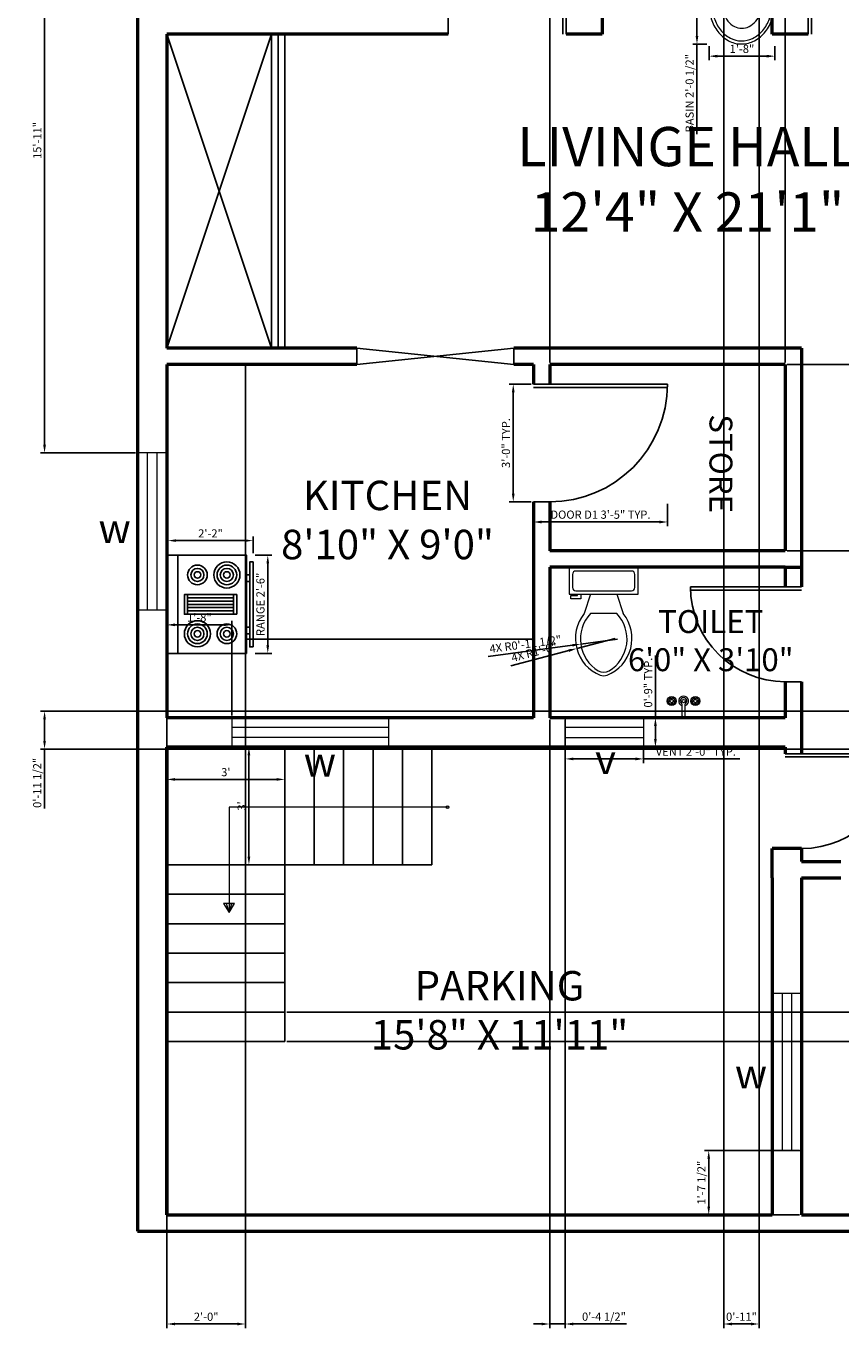
# Model space of a CAD drawing. Units: inches. Extents: x 1962 to 2423, y 2693 to 3296.
# Tile 1 of 4: x 1962 to 2212, y 2693 to 3092. Entities that reach past the tile are written whole.
import ezdxf

# ---------------------------------------------------------------- set-up
doc = ezdxf.new("R2010")
doc.units = ezdxf.units.IN
for name, color, linetype, lineweight in [('A-ANNO-DIMS', 2, 'Continuous', 18), ('A-ANNO-SYMB', 7, 'Continuous', 18), ('A-ANNO-TEXT', 3, 'Continuous', 18), ('A-AREA-IDEN', 7, 'Continuous', 25), ('A-DOOR', 3, 'Continuous', 25), ('A-EQPM', 8, 'Continuous', 25), ('A-FLOR-CASE', 9, 'Continuous', 25), ('A-FLOR-FIXT', 9, 'Continuous', 18), ('A-FLOR-STRS', 7, 'Continuous', 25), ('A-GLAZ', 4, 'Continuous', 18), ('A-WALL', 7, 'Continuous', 50)]:
    doc.layers.add(name, color=color, linetype=linetype, lineweight=lineweight)
doc.styles.get("Standard").update_dxf_attribs({"font": 'arial.ttf'})
doc.dimstyles.new('ISO-25', dxfattribs={"dimtxt": 2.5, "dimasz": 2.5, "dimexe": 1.25, "dimexo": 0.625, "dimtad": 1, "dimdec": 0, "dimlunit": 3, "dimtxsty": 'Standard', "dimcen": 2.5, "dimadec": 0, "dimazin": 0, "dimtfac": 1, "dimtdec": 0, "dimtmove": 0, "dimatfit": 3, "dimfxl": 1, "dimarcsym": 0})

# ---------------------------------------------------------------- blocks, each defined once
blk = doc.blocks.new('Range-Oven - 30 in top')
for p, q in [((0, -3), (30, -3)), ((12, -6), (18, -6)), ((13, -20), (13, -6)), ((14, -6), (14, -20)), ((15, -20), (15, -6)), ((16, -6), (16, -20)), ((17, -20), (17, -6)), ((18, -20), (12, -20)), ((6, -24), (6, -25)), ((8, -25), (8, -24)), ((22, -25), (22, -24)), ((24, -24), (24, -25))]:
    blk.add_line(p, q)
for points in [[(0, -24), (0, 0), (30, 0), (30, -24)], [(12, -21), (12, -5), (18, -5), (18, -21)], [(2, -26), (2, -25), (28, -25), (28, -26)]]:
    blk.add_lwpolyline(points, close=True)
for centre, radius in [((6, -9), 4), ((6, -9), 3), ((6, -9), 2), ((24, -9), 3), ((24, -9), 2), ((6, -9), 1), ((24, -9), 1), ((6, -18), 3), ((24, -18), 4), ((24, -18), 3), ((6, -18), 2), ((6, -18), 1), ((24, -18), 2), ((24, -18), 1)]:
    blk.add_circle(centre, radius)
blk = doc.blocks.new('Sink - Oval top')
for p, q in [((-1, 0), (1, 0)), ((0, 1), (0, -1))]:
    blk.add_line(p, q)
for points in [[(-12.23, 0.39, 0.117634), (-11.46, -3.36, 0.104469), (-8.88, -6.8, 0.090016), (-5.08, -9.07, 0.08192), (-0.32, -10.02, 0.08192), (4.49, -9.38, 0.090016), (8.42, -7.36, 0.104469), (11.22, -4.09, 0.117634), (12.23, -0.39, 0.117634), (11.46, 3.36, 0.104469), (8.88, 6.8, 0.090016), (5.08, 9.07, 0.08192), (0.32, 10.02, 0.08192), (-4.49, 9.38, 0.090016), (-8.42, 7.36, 0.104469), (-11.22, 4.09, 0.117634)], [(-11.29, 0.16, 0.118622), (-10.52, -3.25, 0.104678), (-8.07, -6.36, 0.089562), (-4.54, -8.37, 0.081185), (-0.13, -9.15, 0.081185), (4.3, -8.49, 0.089562), (7.89, -6.58, 0.104678), (10.42, -3.55, 0.118622), (11.29, -0.16, 0.118622), (10.52, 3.25, 0.104678), (8.07, 6.36, 0.089562), (4.54, 8.37, 0.081185), (0.13, 9.15, 0.081185), (-4.3, 8.49, 0.089562), (-7.89, 6.58, 0.104678), (-10.42, 3.55, 0.118622)], [(-7.42, 0.08, 0.118283), (-6.91, -2.17, 0.104607), (-5.29, -4.21, 0.089718), (-2.97, -5.53, 0.081436), (-0.07, -6.04, 0.081436), (2.84, -5.59, 0.089718), (5.2, -4.33, 0.104607), (6.86, -2.32, 0.118283), (7.42, -0.08, 0.118283), (6.91, 2.17, 0.104607), (5.29, 4.21, 0.089718), (2.97, 5.53, 0.081436), (0.07, 6.04, 0.081436), (-2.84, 5.59, 0.089718), (-5.2, 4.33, 0.104607), (-6.86, 2.32, 0.118283)]]:
    blk.add_lwpolyline(points, format="xyb", close=True)
for radius in [1.5, 1]:
    blk.add_circle((0, 0), radius)
blk = doc.blocks.new('Faucet - Bathroom top')
for p, q in [((-4.107, 0.125), (-4.375, 0.125)), ((-3.75, 0.4788), (-3.75, 0.75)), ((-3.5, 0.482), (-3.5, 0.75)), ((-3.1461, 0.125), (-2.875, 0.125)), ((3.143, 0.125), (2.875, 0.125)), ((3.5, 0.4788), (3.5, 0.75)), ((3.75, 0.482), (3.75, 0.75)), ((4.1039, 0.125), (4.375, 0.125)), ((-4.1039, -0.125), (-4.375, -0.125)), ((-3.75, -0.4821), (-3.75, -0.75)), ((-3.5, -0.4789), (-3.5, -0.75)), ((-3.143, -0.125), (-2.875, -0.125)), ((-0.5, -0.8639), (-0.5, -4.5)), ((0.5, -4.5), (0.5, -0.8631)), ((3.1461, -0.125), (2.875, -0.125)), ((3.5, -0.4821), (3.5, -0.75)), ((3.75, -0.4789), (3.75, -0.75)), ((4.107, -0.125), (4.375, -0.125))]:
    blk.add_line(p, q)
for centre, radius in [((-3.625, 0), 1.375), ((-4.625, 0), 0.2795), ((-3.625, 0), 0.5), ((-3.625, 1), 0.2795), ((-2.625, 0), 0.2795), ((0, 0), 0.5), ((3.625, 0), 1.375), ((2.625, 0), 0.2795), ((3.625, 0), 0.5), ((3.625, 1), 0.2795), ((4.625, 0), 0.2795), ((-3.625, -1), 0.2795), ((3.625, -1), 0.2795)]:
    blk.add_circle(centre, radius)
for centre, radius, start, end in [((-3.625, 0), 1, 105.2407, 164.2093), ((-3.625, 0), 1, 16.44125, 74.07887), ((0, 0), 1.5, 289.6514, 250.3603), ((0, 0), 1, 300.3431, 239.7554), ((3.625, 0), 1, 106.12, 164.0884), ((3.625, 0), 1, 16.23422, 73.90469), ((-3.625, 0), 1, 196.2342, 253.9047), ((-3.625, 0), 1, 286.12, 344.0884), ((3.625, 0), 1, 196.4413, 254.0789), ((3.625, 0), 1, 285.2407, 344.2093), ((0, -4.5), 0.5, 180, 0)]:
    blk.add_arc(centre, radius, start, end)
blk = doc.blocks.new('Toilet - top')
for p, q in [((9.5, -6), (9.5, -2)), ((-10, -8.5), (-8, -8.5)), ((-10, -9.5), (-10, -8.5)), ((-7, -9.5), (-10, -9.5)), ((-8, -8.5), (-8, -8)), ((-7, -8), (-7, -9.5)), ((-4, -8), (-6, -14)), ((4, -8), (6, -14)), ((4, -14), (-4, -14))]:
    blk.add_line(p, q)
blk.add_lwpolyline([(10.5, -8), (10.5, 0), (-10.5, 0), (-10.5, -8)], close=True)
for points in [[(-9.5, -2), (-9.5, -6)], [(8.5, -1), (-8.5, -1)], [(-8.5, -7), (8.5, -7)]]:
    blk.add_lwpolyline(points)
for centre, radius, start, end in [((-8.62, -1.88), 0.884, 81.8699, 188.1301), ((8.62, -1.88), 0.884, 351.8699, 98.1301), ((-8.62, -6.12), 0.884, 171.8699, 278.1301), ((8.62, -6.12), 0.884, 261.8699, 8.1301), ((3.52, -21.58), 12.17, 141.4691, 247.9714), ((4.2, -21.82), 11.33, 136.3677, 238.9468), ((-3.52, -21.58), 12.17, 292.0284, 38.5307), ((-4.2, -21.82), 11.33, 301.053, 43.6321), ((0, -27.88), 4, 245.7318, 294.2682), ((0, -29), 4, 254.8605, 285.1395)]:
    blk.add_arc(centre, radius, start, end)
blk = doc.blocks.new('*D15')
at = {"layer": 'A-ANNO-DIMS', "color": 0, "lineweight": -2, "transparency": 16777216}
for p, q in [((2005.54, 2870.96), (2005.54, 2860.47)), ((2041.54, 2870.96), (2041.54, 2860.47)), ((2008.04, 2861.72), (2039.04, 2861.72))]:
    blk.add_line(p, q, dxfattribs=at)
at = {"layer": 'A-ANNO-DIMS', "color": 0, "transparency": 16777216}
for points in [[(2008.04, 2862.14), (2008.04, 2861.3), (2005.54, 2861.72)], [(2039.04, 2862.14), (2039.04, 2861.3), (2041.54, 2861.72)]]:
    blk.add_solid(points, dxfattribs=at)
at = {"layer": 'Defpoints', "color": 0, "transparency": 16777216}
for p in [(2005.54, 2871.59), (2041.54, 2871.59), (2041.54, 2861.72)]:
    blk.add_point(p, dxfattribs=at)
at = {"layer": 'A-ANNO-DIMS', "color": 0, "transparency": 16777216, "insert": (2023.54, 2863.62), "char_height": 2.5, "attachment_point": 5}
blk.add_mtext("3'", dxfattribs=at)
blk = doc.blocks.new('*D16')
at = {"layer": 'A-ANNO-DIMS', "color": 0, "lineweight": -2, "transparency": 16777216}
for p, q in [((2040.91, 2871.59), (2029.35, 2871.59)), ((2030.6, 2869.09), (2030.6, 2838.09)), ((2040.91, 2835.59), (2029.35, 2835.59))]:
    blk.add_line(p, q, dxfattribs=at)
at = {"layer": 'A-ANNO-DIMS', "color": 0, "transparency": 16777216}
for points in [[(2030.19, 2869.09), (2031.02, 2869.09), (2030.6, 2871.59)], [(2030.19, 2838.09), (2031.02, 2838.09), (2030.6, 2835.59)]]:
    blk.add_solid(points, dxfattribs=at)
at = {"layer": 'Defpoints', "color": 0, "transparency": 16777216}
for p in [(2041.54, 2871.59), (2030.6, 2835.59), (2041.54, 2835.59)]:
    blk.add_point(p, dxfattribs=at)
at = {"layer": 'A-ANNO-DIMS', "color": 0, "transparency": 16777216, "insert": (2028.7, 2853.59), "char_height": 2.5, "attachment_point": 5, "rotation": 90}
blk.add_mtext("3'", dxfattribs=at)
blk = doc.blocks.new('DOOR-SWING-36IN')
for p, q in [((0, 5), (0, 41)), ((1, 5), (1, 41)), ((0, 5), (0, 0)), ((1, 5), (1, 0)), ((36, 0), (36, 5))]:
    blk.add_line(p, q)
blk.add_arc((0, 5), 36, 0, 90)
blk = doc.blocks.new('DOOR-SWING-29IN')
for p, q in [((0, 5), (0, 34)), ((1, 5), (1, 34)), ((0, 5), (0, 0)), ((1, 5), (1, 0)), ((29, 0), (29, 5))]:
    blk.add_line(p, q)
blk.add_arc((0, 5), 29, 0, 90)
blk = doc.blocks.new('WINDOW-48IN')
for p, q in [((0, 48), (0, 0)), ((9, 48), (0, 48)), ((3, 48), (3, 0)), ((6, 0), (6, 48)), ((9, 0), (9, 48)), ((0, 0), (9, 0))]:
    blk.add_line(p, q)
blk = doc.blocks.new('VENT-24IN')
for p, q in [((24, 9), (0, 9)), ((0, 9), (0, 0)), ((24, 9), (24, 0)), ((24, 6), (0, 6)), ((0, 3), (24, 3)), ((0, 0), (24, 0))]:
    blk.add_line(p, q)
blk = doc.blocks.new('*D26')
at = {"layer": 'A-ANNO-DIMS', "color": 0, "lineweight": -2, "transparency": 16777216}
for p, q in [((2117.54, 2945.96), (2117.54, 2939.19)), ((2158.54, 2945.96), (2158.54, 2939.19)), ((2120.04, 2940.44), (2156.04, 2940.44))]:
    blk.add_line(p, q, dxfattribs=at)
at = {"layer": 'A-ANNO-DIMS', "color": 0, "transparency": 16777216}
for points in [[(2120.04, 2940.86), (2120.04, 2940.02), (2117.54, 2940.44)], [(2156.04, 2940.86), (2156.04, 2940.02), (2158.54, 2940.44)]]:
    blk.add_solid(points, dxfattribs=at)
at = {"layer": 'Defpoints', "color": 0, "transparency": 16777216}
for p in [(2117.54, 2946.59), (2158.54, 2946.59), (2158.54, 2940.44)]:
    blk.add_point(p, dxfattribs=at)
at = {"layer": 'A-ANNO-DIMS', "color": 0, "transparency": 16777216, "insert": (2138.04, 2942.36), "char_height": 2.5, "attachment_point": 5}
blk.add_mtext('DOOR D1 3\'-5" TYP.', dxfattribs=at)
blk = doc.blocks.new('*D27')
at = {"layer": 'A-ANNO-DIMS', "color": 0, "lineweight": -2, "transparency": 16777216}
for p, q in [((2116.91, 2982.59), (2110.14, 2982.59)), ((2111.39, 2980.09), (2111.39, 2949.09)), ((2116.91, 2946.59), (2110.14, 2946.59))]:
    blk.add_line(p, q, dxfattribs=at)
at = {"layer": 'A-ANNO-DIMS', "color": 0, "transparency": 16777216}
for points in [[(2110.97, 2980.09), (2111.8, 2980.09), (2111.39, 2982.59)], [(2110.97, 2949.09), (2111.8, 2949.09), (2111.39, 2946.59)]]:
    blk.add_solid(points, dxfattribs=at)
at = {"layer": 'Defpoints', "color": 0, "transparency": 16777216}
for p in [(2117.54, 2982.59), (2111.39, 2946.59), (2117.54, 2946.59)]:
    blk.add_point(p, dxfattribs=at)
at = {"layer": 'A-ANNO-DIMS', "color": 0, "transparency": 16777216, "insert": (2109.48, 2964.59), "char_height": 2.5, "attachment_point": 5, "rotation": 90}
blk.add_mtext('3\'-0" TYP.', dxfattribs=at)
blk = doc.blocks.new('*D38')
at = {"layer": 'A-ANNO-DIMS', "color": 0, "lineweight": -2, "transparency": 16777216}
for p, q in [((2127.24, 2870.96), (2127.24, 2866.74)), ((2151.24, 2870.96), (2151.24, 2866.74)), ((2129.74, 2867.99), (2148.74, 2867.99)), ((2151.24, 2867.99), (2180.65, 2867.99))]:
    blk.add_line(p, q, dxfattribs=at)
at = {"layer": 'A-ANNO-DIMS', "color": 0, "transparency": 16777216}
for points in [[(2129.74, 2868.41), (2129.74, 2867.57), (2127.24, 2867.99)], [(2148.74, 2868.41), (2148.74, 2867.57), (2151.24, 2867.99)]]:
    blk.add_solid(points, dxfattribs=at)
at = {"layer": 'Defpoints', "color": 0, "transparency": 16777216}
for p in [(2127.24, 2871.59), (2151.24, 2871.59), (2151.24, 2867.99)]:
    blk.add_point(p, dxfattribs=at)
at = {"layer": 'A-ANNO-DIMS', "color": 0, "transparency": 16777216, "insert": (2167.2, 2869.89), "char_height": 2.5, "attachment_point": 5}
blk.add_mtext('VENT 2\'-0" TYP.', dxfattribs=at)
blk = doc.blocks.new('*D39')
at = {"layer": 'A-ANNO-DIMS', "color": 0, "lineweight": -2, "transparency": 16777216}
for p, q in [((2154.84, 2880.59), (2154.84, 2899.58)), ((2151.87, 2880.59), (2156.09, 2880.59)), ((2154.84, 2874.09), (2154.84, 2878.09)), ((2151.87, 2871.59), (2156.09, 2871.59))]:
    blk.add_line(p, q, dxfattribs=at)
at = {"layer": 'A-ANNO-DIMS', "color": 0, "transparency": 16777216}
for points in [[(2154.43, 2878.09), (2155.26, 2878.09), (2154.84, 2880.59)], [(2154.43, 2874.09), (2155.26, 2874.09), (2154.84, 2871.59)]]:
    blk.add_solid(points, dxfattribs=at)
at = {"layer": 'Defpoints', "color": 0, "transparency": 16777216}
for p in [(2151.24, 2880.59), (2154.84, 2880.59), (2151.24, 2871.59)]:
    blk.add_point(p, dxfattribs=at)
at = {"layer": 'A-ANNO-DIMS', "color": 0, "transparency": 16777216, "insert": (2152.94, 2891.33), "char_height": 2.5, "attachment_point": 5, "rotation": 90}
blk.add_mtext('0\'-9" TYP.', dxfattribs=at)
blk = doc.blocks.new('*D40')
at = {"layer": 'A-ANNO-DIMS', "color": 0, "lineweight": -2, "transparency": 16777216}
for p, q in [((2032.48, 2930.25), (2037.61, 2930.25)), ((2036.36, 2902.75), (2036.36, 2927.75)), ((2032.48, 2900.25), (2037.61, 2900.25))]:
    blk.add_line(p, q, dxfattribs=at)
at = {"layer": 'A-ANNO-DIMS', "color": 0, "transparency": 16777216}
for points in [[(2035.94, 2927.75), (2036.78, 2927.75), (2036.36, 2930.25)], [(2035.94, 2902.75), (2036.78, 2902.75), (2036.36, 2900.25)]]:
    blk.add_solid(points, dxfattribs=at)
at = {"layer": 'Defpoints', "color": 0, "transparency": 16777216}
for p in [(2031.86, 2930.25), (2036.36, 2930.25), (2031.86, 2900.25)]:
    blk.add_point(p, dxfattribs=at)
at = {"layer": 'A-ANNO-DIMS', "color": 0, "transparency": 16777216, "insert": (2034.44, 2915.25), "char_height": 2.5, "attachment_point": 5, "rotation": 90}
blk.add_mtext('RANGE 2\'-6"', dxfattribs=at)
blk = doc.blocks.new('*D41')
at = {"layer": 'A-ANNO-DIMS', "color": 0, "lineweight": -2, "transparency": 16777216}
for p, q in [((2005.86, 2930.88), (2005.86, 2936)), ((2029.36, 2934.75), (2008.36, 2934.75)), ((2031.86, 2930.88), (2031.86, 2936))]:
    blk.add_line(p, q, dxfattribs=at)
at = {"layer": 'A-ANNO-DIMS', "color": 0, "transparency": 16777216}
for points in [[(2008.36, 2935.17), (2008.36, 2934.34), (2005.86, 2934.75)], [(2029.36, 2935.17), (2029.36, 2934.34), (2031.86, 2934.75)]]:
    blk.add_solid(points, dxfattribs=at)
at = {"layer": 'Defpoints', "color": 0, "transparency": 16777216}
for p in [(2005.86, 2934.75), (2005.86, 2930.25), (2031.86, 2930.25)]:
    blk.add_point(p, dxfattribs=at)
at = {"layer": 'A-ANNO-DIMS', "color": 0, "transparency": 16777216, "insert": (2018.86, 2936.63), "char_height": 2.5, "attachment_point": 5}
blk.add_mtext('2\'-2"', dxfattribs=at)
blk = doc.blocks.new('*D48')
at = {"layer": 'A-ANNO-DIMS', "color": 0, "lineweight": -2, "transparency": 16777216}
for p, q in [((2170.6, 3111.12), (2166.29, 3111.12)), ((2167.54, 3108.62), (2167.54, 3089.07)), ((2170.6, 3086.57), (2166.29, 3086.57)), ((2167.54, 3086.57), (2167.54, 3059.01))]:
    blk.add_line(p, q, dxfattribs=at)
at = {"layer": 'A-ANNO-DIMS', "color": 0, "transparency": 16777216}
for points in [[(2167.12, 3108.62), (2167.96, 3108.62), (2167.54, 3111.12)], [(2167.12, 3089.07), (2167.96, 3089.07), (2167.54, 3086.57)]]:
    blk.add_solid(points, dxfattribs=at)
at = {"layer": 'Defpoints', "color": 0, "transparency": 16777216}
for p in [(2171.22, 3111.12), (2167.54, 3086.57), (2171.22, 3086.57)]:
    blk.add_point(p, dxfattribs=at)
at = {"layer": 'A-ANNO-DIMS', "color": 0, "transparency": 16777216, "insert": (2165.62, 3071.54), "char_height": 2.5, "attachment_point": 5, "rotation": 90}
blk.add_mtext('BASIN 2\'-0 1/2"', dxfattribs=at)
blk = doc.blocks.new('*D49')
at = {"layer": 'A-ANNO-DIMS', "color": 0, "lineweight": -2, "transparency": 16777216}
for p, q in [((2171.22, 3085.94), (2171.22, 3081.64)), ((2173.72, 3082.89), (2188.86, 3082.89)), ((2191.36, 3085.94), (2191.36, 3081.64))]:
    blk.add_line(p, q, dxfattribs=at)
at = {"layer": 'A-ANNO-DIMS', "color": 0, "transparency": 16777216}
for points in [[(2173.72, 3083.3), (2173.72, 3082.47), (2171.22, 3082.89)], [(2188.86, 3083.3), (2188.86, 3082.47), (2191.36, 3082.89)]]:
    blk.add_solid(points, dxfattribs=at)
at = {"layer": 'Defpoints', "color": 0, "transparency": 16777216}
for p in [(2171.22, 3086.57), (2191.36, 3086.57), (2191.36, 3082.89)]:
    blk.add_point(p, dxfattribs=at)
at = {"layer": 'A-ANNO-DIMS', "color": 0, "transparency": 16777216, "insert": (2181.29, 3084.79), "char_height": 2.5, "attachment_point": 5}
blk.add_mtext('1\'-8"', dxfattribs=at)
blk = doc.blocks.new('*D52')
at = {"layer": 'A-ANNO-DIMS', "color": 0, "lineweight": -2, "transparency": 16777216}
for p, q in [((2195.16, 2988.59), (2386.19, 2988.59)), ((2384.94, 2934.09), (2384.94, 2986.09)), ((2195.16, 2931.59), (2386.19, 2931.59))]:
    blk.add_line(p, q, dxfattribs=at)
at = {"layer": 'A-ANNO-DIMS', "color": 0, "transparency": 16777216}
for points in [[(2384.52, 2986.09), (2385.35, 2986.09), (2384.94, 2988.59)], [(2384.52, 2934.09), (2385.35, 2934.09), (2384.94, 2931.59)]]:
    blk.add_solid(points, dxfattribs=at)
at = {"layer": 'Defpoints', "color": 0, "transparency": 16777216}
for p in [(2194.54, 2988.59), (2384.94, 2988.59), (2194.54, 2931.59)]:
    blk.add_point(p, dxfattribs=at)
at = {"layer": 'A-ANNO-DIMS', "color": 0, "transparency": 16777216, "insert": (2383.04, 2960.09), "char_height": 2.5, "attachment_point": 5, "rotation": 90}
blk.add_mtext('4\'-9"', dxfattribs=at)
blk = doc.blocks.new('*D53')
at = {"layer": 'A-ANNO-DIMS', "color": 0, "lineweight": -2, "transparency": 16777216}
for p, q in [((2122.54, 2989.21), (2122.54, 3293.29)), ((2125.04, 3292.04), (2192.04, 3292.04)), ((2194.54, 2989.21), (2194.54, 3293.29))]:
    blk.add_line(p, q, dxfattribs=at)
at = {"layer": 'A-ANNO-DIMS', "color": 0, "transparency": 16777216}
for points in [[(2125.04, 3292.46), (2125.04, 3291.63), (2122.54, 3292.04)], [(2192.04, 3292.46), (2192.04, 3291.63), (2194.54, 3292.04)]]:
    blk.add_solid(points, dxfattribs=at)
at = {"layer": 'Defpoints', "color": 0, "transparency": 16777216}
for p in [(2194.54, 3292.04), (2122.54, 2988.59), (2194.54, 2988.59)]:
    blk.add_point(p, dxfattribs=at)
at = {"layer": 'A-ANNO-DIMS', "color": 0, "transparency": 16777216, "insert": (2158.54, 3293.94), "char_height": 2.5, "attachment_point": 5}
blk.add_mtext('6\'-0"', dxfattribs=at)
blk = doc.blocks.new('*D63')
at = {"layer": 'A-ANNO-DIMS', "color": 0, "lineweight": -2, "transparency": 16777216}
for p, q in [((1995.91, 3152.67), (1966.89, 3152.67)), ((1968.14, 2964.06), (1968.14, 3150.17)), ((1995.91, 2961.56), (1966.89, 2961.56))]:
    blk.add_line(p, q, dxfattribs=at)
at = {"layer": 'A-ANNO-DIMS', "color": 0, "transparency": 16777216}
for points in [[(1967.72, 3150.17), (1968.55, 3150.17), (1968.14, 3152.67)], [(1967.72, 2964.06), (1968.55, 2964.06), (1968.14, 2961.56)]]:
    blk.add_solid(points, dxfattribs=at)
at = {"layer": 'Defpoints', "color": 0, "transparency": 16777216}
for p in [(1968.14, 3152.67), (1996.54, 3152.67), (1996.54, 2961.56)]:
    blk.add_point(p, dxfattribs=at)
at = {"layer": 'A-ANNO-DIMS', "color": 0, "transparency": 16777216, "insert": (1966.24, 3057.11), "char_height": 2.5, "attachment_point": 5, "rotation": 90}
blk.add_mtext('15\'-11"', dxfattribs=at)
blk = doc.blocks.new('*D64')
at = {"layer": 'A-ANNO-DIMS', "color": 0, "lineweight": -2, "transparency": 16777216}
for p, q in [((2005.54, 2987.96), (2005.54, 2693.94)), ((2029.54, 2987.96), (2029.54, 2693.94)), ((2008.04, 2695.19), (2027.04, 2695.19))]:
    blk.add_line(p, q, dxfattribs=at)
at = {"layer": 'A-ANNO-DIMS', "color": 0, "transparency": 16777216}
for points in [[(2008.04, 2695.61), (2008.04, 2694.77), (2005.54, 2695.19)], [(2027.04, 2695.61), (2027.04, 2694.77), (2029.54, 2695.19)]]:
    blk.add_solid(points, dxfattribs=at)
at = {"layer": 'Defpoints', "color": 0, "transparency": 16777216}
for p in [(2005.54, 2988.59), (2029.54, 2988.59), (2029.54, 2695.19)]:
    blk.add_point(p, dxfattribs=at)
at = {"layer": 'A-ANNO-DIMS', "color": 0, "transparency": 16777216, "insert": (2017.54, 2697.09), "char_height": 2.5, "attachment_point": 5}
blk.add_mtext('2\'-0"', dxfattribs=at)
blk = doc.blocks.new('*D66')
at = {"layer": 'A-ANNO-DIMS', "color": 0, "lineweight": -2, "transparency": 16777216}
for p, q in [((2270.96, 2882.58), (1966.89, 2882.58)), ((1968.14, 2880.08), (1968.14, 2873.51)), ((2262.7, 2871.01), (1966.89, 2871.01)), ((1968.14, 2871.01), (1968.14, 2852.84))]:
    blk.add_line(p, q, dxfattribs=at)
at = {"layer": 'A-ANNO-DIMS', "color": 0, "transparency": 16777216}
for points in [[(1967.72, 2880.08), (1968.55, 2880.08), (1968.14, 2882.58)], [(1967.72, 2873.51), (1968.55, 2873.51), (1968.14, 2871.01)]]:
    blk.add_solid(points, dxfattribs=at)
at = {"layer": 'Defpoints', "color": 0, "transparency": 16777216}
for p in [(2271.59, 2882.58), (1968.14, 2871.01), (2263.33, 2871.01)]:
    blk.add_point(p, dxfattribs=at)
at = {"layer": 'A-ANNO-DIMS', "color": 0, "transparency": 16777216, "insert": (1966.22, 2860.67), "char_height": 2.5, "attachment_point": 5, "rotation": 90}
blk.add_mtext('0\'-11 1/2"', dxfattribs=at)
blk = doc.blocks.new('*D67')
at = {"layer": 'A-ANNO-DIMS', "color": 0, "lineweight": -2, "transparency": 16777216}
for p, q in [((2198.91, 2748.21), (2169.89, 2748.21)), ((2171.14, 2731.09), (2171.14, 2745.71)), ((2198.91, 2728.59), (2169.89, 2728.59))]:
    blk.add_line(p, q, dxfattribs=at)
at = {"layer": 'A-ANNO-DIMS', "color": 0, "transparency": 16777216}
for points in [[(2170.72, 2745.71), (2171.55, 2745.71), (2171.14, 2748.21)], [(2170.72, 2731.09), (2171.55, 2731.09), (2171.14, 2728.59)]]:
    blk.add_solid(points, dxfattribs=at)
at = {"layer": 'Defpoints', "color": 0, "transparency": 16777216}
for p in [(2171.14, 2748.21), (2199.54, 2748.21), (2199.54, 2728.59)]:
    blk.add_point(p, dxfattribs=at)
at = {"layer": 'A-ANNO-DIMS', "color": 0, "transparency": 16777216, "insert": (2169.22, 2738.4), "char_height": 2.5, "attachment_point": 5, "rotation": 90}
blk.add_mtext('1\'-7 1/2"', dxfattribs=at)
blk = doc.blocks.new('*D68')
at = {"layer": 'A-ANNO-DIMS', "color": 0, "lineweight": -2, "transparency": 16777216}
for p, q in [((2005.54, 2881.21), (2005.51, 2910.24)), ((2008.02, 2908.99), (2022.88, 2909)), ((2025.4, 2881.23), (2025.38, 2910.25))]:
    blk.add_line(p, q, dxfattribs=at)
at = {"layer": 'A-ANNO-DIMS', "color": 0, "transparency": 16777216}
for points in [[(2008.01, 2909.41), (2008.02, 2908.57), (2005.52, 2908.99)], [(2022.88, 2909.42), (2022.88, 2908.59), (2025.38, 2909)]]:
    blk.add_solid(points, dxfattribs=at)
at = {"layer": 'Defpoints', "color": 0, "transparency": 16777216}
for p in [(2025.38, 2909), (2005.54, 2880.59), (2025.4, 2880.6)]:
    blk.add_point(p, dxfattribs=at)
at = {"layer": 'A-ANNO-DIMS', "color": 0, "transparency": 16777216, "insert": (2015.45, 2910.9), "char_height": 2.5, "attachment_point": 5, "rotation": 0.0435}
blk.add_mtext('1\'-8"', dxfattribs=at)
blk = doc.blocks.new('*D69')
at = {"layer": 'A-ANNO-DIMS', "color": 0, "lineweight": -2, "transparency": 16777216}
for p, q in [((2042.16, 2790.59), (2386.19, 2790.59)), ((2384.94, 2784.09), (2384.94, 2788.09)), ((2042.16, 2781.59), (2386.19, 2781.59))]:
    blk.add_line(p, q, dxfattribs=at)
at = {"layer": 'A-ANNO-DIMS', "color": 0, "transparency": 16777216}
for points in [[(2384.52, 2788.09), (2385.35, 2788.09), (2384.94, 2790.59)], [(2384.52, 2784.09), (2385.35, 2784.09), (2384.94, 2781.59)]]:
    blk.add_solid(points, dxfattribs=at)
at = {"layer": 'Defpoints', "color": 0, "transparency": 16777216}
for p in [(2041.54, 2790.59), (2384.94, 2790.59), (2041.54, 2781.59)]:
    blk.add_point(p, dxfattribs=at)
at = {"layer": 'A-ANNO-DIMS', "color": 0, "transparency": 16777216, "insert": (2383.04, 2786.09), "char_height": 2.5, "attachment_point": 5, "rotation": 90}
blk.add_mtext('0\'-9"', dxfattribs=at)
blk = doc.blocks.new('*D70')
at = {"layer": 'A-ANNO-DIMS', "color": 0, "lineweight": -2, "transparency": 16777216}
for p, q in [((2122.54, 2879.96), (2122.54, 2693.94)), ((2127.24, 2879.96), (2127.24, 2693.94)), ((2120.04, 2695.19), (2117.54, 2695.19)), ((2122.54, 2695.19), (2127.24, 2695.19)), ((2129.74, 2695.19), (2145.97, 2695.19))]:
    blk.add_line(p, q, dxfattribs=at)
at = {"layer": 'A-ANNO-DIMS', "color": 0, "transparency": 16777216}
for points in [[(2120.04, 2695.61), (2120.04, 2694.77), (2122.54, 2695.19)], [(2129.74, 2695.61), (2129.74, 2694.77), (2127.24, 2695.19)]]:
    blk.add_solid(points, dxfattribs=at)
at = {"layer": 'Defpoints', "color": 0, "transparency": 16777216}
for p in [(2122.54, 2880.59), (2127.24, 2880.59), (2127.24, 2695.19)]:
    blk.add_point(p, dxfattribs=at)
at = {"layer": 'A-ANNO-DIMS', "color": 0, "transparency": 16777216, "insert": (2139.11, 2697.11), "char_height": 2.5, "attachment_point": 5}
blk.add_mtext('0\'-4 1/2"', dxfattribs=at)
blk = doc.blocks.new('*D71')
at = {"layer": 'A-ANNO-DIMS', "color": 0, "lineweight": -2, "transparency": 16777216}
for p, q in [((2175.74, 3214.96), (2175.74, 2693.94)), ((2186.54, 3214.96), (2186.54, 2693.94)), ((2184.04, 2695.19), (2178.24, 2695.19))]:
    blk.add_line(p, q, dxfattribs=at)
at = {"layer": 'A-ANNO-DIMS', "color": 0, "transparency": 16777216}
for points in [[(2178.24, 2695.61), (2178.24, 2694.77), (2175.74, 2695.19)], [(2184.04, 2695.61), (2184.04, 2694.77), (2186.54, 2695.19)]]:
    blk.add_solid(points, dxfattribs=at)
at = {"layer": 'Defpoints', "color": 0, "transparency": 16777216}
for p in [(2175.74, 3215.59), (2186.54, 3215.59), (2175.74, 2695.19)]:
    blk.add_point(p, dxfattribs=at)
at = {"layer": 'A-ANNO-DIMS', "color": 0, "transparency": 16777216, "insert": (2181.14, 2697.09), "char_height": 2.5, "attachment_point": 5}
blk.add_mtext('0\'-11"', dxfattribs=at)
blk = doc.blocks.new('*D76')
at = {"layer": 'A-ANNO-DIMS', "color": 0, "lineweight": -2, "transparency": 16777216}
for p, q in [((2142.55, 2904.84), (2130.78, 2901.75)), ((2110.7, 2896.48), (2128.36, 2901.12))]:
    blk.add_line(p, q, dxfattribs=at)
at = {"layer": 'A-ANNO-DIMS', "color": 0, "transparency": 16777216}
blk.add_solid([(2128.25, 2901.52), (2128.47, 2900.71), (2130.78, 2901.75)], dxfattribs=at)
at = {"layer": 'Defpoints', "color": 0, "transparency": 16777216}
for p in [(2142.55, 2904.84), (2130.78, 2901.75)]:
    blk.add_point(p, dxfattribs=at)
at = {"layer": 'A-ANNO-DIMS', "color": 0, "transparency": 16777216, "insert": (2117.84, 2900.32), "char_height": 2.5, "attachment_point": 5, "rotation": 14.7215}
blk.add_mtext('4X R1\'-0"', dxfattribs=at)
blk = doc.blocks.new('*D77')
at = {"layer": 'A-ANNO-DIMS', "color": 0, "lineweight": -2, "transparency": 16777216}
for p, q in [((2103.73, 2899.3), (2129.52, 2902.76)), ((2143.23, 2904.61), (2132, 2903.1))]:
    blk.add_line(p, q, dxfattribs=at)
at = {"layer": 'A-ANNO-DIMS', "color": 0, "transparency": 16777216}
blk.add_solid([(2129.47, 2903.18), (2129.58, 2902.35), (2132, 2903.1)], dxfattribs=at)
at = {"layer": 'Defpoints', "color": 0, "transparency": 16777216}
for p in [(2132, 2903.1), (2143.23, 2904.61)]:
    blk.add_point(p, dxfattribs=at)
at = {"layer": 'A-ANNO-DIMS', "color": 0, "transparency": 16777216, "insert": (2115.13, 2902.76), "char_height": 2.5, "attachment_point": 5, "rotation": 7.6568}
blk.add_mtext('4X R0\'-11 1/2"', dxfattribs=at)

msp = doc.modelspace()

# ---------------------------------------------------------------- linework, layer by layer
at = {"layer": 'A-ANNO-SYMB'}
for p, q in [((2091.29, 2853.23), (2024.53, 2853.23)), ((2024.53, 2853.23), (2024.53, 2823.81)), ((2026.22, 2823.81), (2022.79, 2823.81)), ((2022.79, 2823.81), (2024.58, 2821.04)), ((2024.58, 2821.04), (2023.7, 2823.81)), ((2024.53, 2823.81), (2026.22, 2823.81)), ((2024.53, 2823.81), (2024.58, 2821.04)), ((2024.58, 2821.04), (2026.22, 2823.81)), ((2024.58, 2821.04), (2025.37, 2823.81))]:
    msp.add_line(p, q, dxfattribs=at)
msp.add_circle((2091.29, 2853.23), 0.44, dxfattribs=at)
at = {"layer": 'A-DOOR'}
for p, q in [((2063.54, 2988.59), (2063.54, 2993.59)), ((2063.54, 2988.59), (2111.54, 2993.59)), ((2111.54, 2988.59), (2063.54, 2993.59)), ((2111.54, 2988.59), (2111.54, 2993.59)), ((2111.54, 2993.59), (2111.54, 2988.59)), ((2111.54, 2993.59), (2111.54, 2988.59)), ((2117.54, 2982.59), (2122.54, 2982.59)), ((2199.54, 2920.59), (2194.54, 2920.59)), ((2194.54, 2869.59), (2199.54, 2869.59))]:
    msp.add_line(p, q, dxfattribs=at)
at = {"layer": 'A-FLOR-CASE'}
for p, q in [((2037.54, 3089.59), (2005.54, 2993.59)), ((2005.54, 2993.59), (2005.54, 3089.59)), ((2005.54, 3089.59), (2037.54, 2993.59)), ((2037.54, 3089.59), (2037.54, 2993.59)), ((2039.54, 3089.59), (2039.54, 2993.59)), ((2041.54, 3089.59), (2041.54, 2993.59)), ((2029.54, 2988.59), (2029.54, 2900.25)), ((2117.54, 2904.59), (2029.54, 2904.59)), ((2029.54, 2880.6), (2029.54, 2880.59))]:
    msp.add_line(p, q, dxfattribs=at)
at = {"layer": 'A-FLOR-STRS'}
for p, q in [((2041.54, 2871.59), (2041.54, 2781.59)), ((2050.54, 2871.59), (2050.54, 2835.59)), ((2059.54, 2871.59), (2059.54, 2835.59)), ((2068.54, 2871.59), (2068.54, 2835.59)), ((2077.54, 2871.59), (2077.54, 2835.59)), ((2086.54, 2871.59), (2086.54, 2835.59)), ((2086.54, 2835.59), (2005.54, 2835.59)), ((2041.54, 2826.59), (2005.54, 2826.59)), ((2041.54, 2817.59), (2005.54, 2817.59)), ((2041.54, 2808.59), (2005.54, 2808.59)), ((2041.54, 2799.59), (2005.54, 2799.59)), ((2041.54, 2790.59), (2005.54, 2790.59)), ((2041.54, 2781.59), (2005.54, 2781.59))]:
    msp.add_line(p, q, dxfattribs=at)
at = {"layer": 'A-WALL'}
for p, q in [((1996.54, 3263.59), (1996.54, 2723.59)), ((2138.54, 3110.59), (2138.54, 3089.59)), ((2190.54, 3089.59), (2190.54, 3110.59)), ((2005.54, 3089.59), (2005.54, 2993.59)), ((2091.54, 3089.59), (2005.54, 3089.59)), ((2138.54, 3089.59), (2127.54, 3089.59)), ((2201.54, 3089.59), (2190.54, 3089.59)), ((2063.54, 2993.59), (2005.54, 2993.59)), ((2199.54, 2993.59), (2111.54, 2993.59)), ((2199.54, 2993.59), (2199.54, 2920.59)), ((2005.54, 2988.59), (2005.54, 2880.59)), ((2063.54, 2988.59), (2005.54, 2988.59)), ((2117.54, 2988.59), (2111.54, 2988.59)), ((2117.54, 2988.59), (2111.54, 2988.59)), ((2117.54, 2988.59), (2117.54, 2982.59)), ((2117.54, 2988.59), (2117.54, 2982.59)), ((2122.54, 2988.59), (2122.54, 2982.59)), ((2194.54, 2988.59), (2122.54, 2988.59)), ((2194.54, 2988.59), (2194.54, 2931.59)), ((2117.54, 2946.59), (2117.54, 2880.59)), ((2122.54, 2946.59), (2122.54, 2931.59)), ((2194.54, 2931.59), (2122.54, 2931.59)), ((2194.54, 2926.59), (2122.54, 2926.59)), ((2122.54, 2926.59), (2122.54, 2912.59)), ((2194.54, 2926.59), (2194.54, 2920.59)), ((2194.54, 2926.59), (2199.54, 2926.59)), ((2199.54, 2926.59), (2199.54, 2920.59)), ((2122.54, 2912.59), (2122.54, 2907.59)), ((2122.54, 2907.59), (2122.54, 2880.59)), ((2194.54, 2891.59), (2194.54, 2880.59)), ((2199.54, 2891.59), (2199.54, 2869.59)), ((2117.54, 2880.59), (2005.54, 2880.59)), ((2194.54, 2880.59), (2122.54, 2880.59)), ((2005.54, 2871.59), (2005.54, 2728.59)), ((2117.54, 2871.59), (2005.54, 2871.59)), ((2005.54, 2871.59), (2005.54, 2728.59)), ((2005.54, 2728.59), (2005.54, 2871.59)), ((2122.54, 2871.59), (2117.54, 2871.59)), ((2194.54, 2871.59), (2122.54, 2871.59)), ((2194.54, 2871.59), (2194.54, 2869.59)), ((2194.54, 2871.59), (2194.54, 2869.59)), ((2199.54, 2840.59), (2190.54, 2840.59)), ((2190.54, 2831.59), (2190.54, 2840.59)), ((2199.54, 2840.59), (2199.54, 2836.59)), ((2199.54, 2836.59), (2211.54, 2836.59)), ((2190.54, 2831.59), (2190.54, 2728.59)), ((2199.54, 2831.59), (2211.54, 2831.59)), ((2199.54, 2831.59), (2199.54, 2728.59)), ((2199.54, 2831.59), (2199.54, 2831.59)), ((2199.54, 2831.59), (2211.54, 2831.59)), ((2005.54, 2728.59), (2190.54, 2728.59)), ((2199.54, 2728.59), (2347.54, 2728.59)), ((1996.54, 2723.59), (2356.54, 2723.59))]:
    msp.add_line(p, q, dxfattribs=at)

# ---------------------------------------------------------------- block references
at = {"layer": 'A-DOOR', "extrusion": (0, 0, -1), "zscale": -1}
msp.add_blockref('DOOR-SWING-36IN', (-2127.54, 3089.59), dxfattribs=at)
at = {"layer": 'A-DOOR'}
msp.add_blockref('DOOR-SWING-36IN', (2201.54, 3089.59), dxfattribs=at)
for name, p, rotation in [('DOOR-SWING-36IN', (2117.54, 2982.59), 269.9999999999991), ('DOOR-SWING-29IN', (2194.54, 2869.59), 270.0000000000013)]:
    msp.add_blockref(name, p, dxfattribs=dict(at, rotation=rotation))
at = {"layer": 'A-DOOR', "extrusion": (0, 0, -1), "zscale": -1, "rotation": 270.0000000000001}
msp.add_blockref('DOOR-SWING-29IN', (-2199.54, 2920.59), dxfattribs=at)
at = {"layer": 'A-EQPM', "rotation": 90}
msp.add_blockref('Range-Oven - 30 in top', (2005.86, 2900.25), dxfattribs=at)
at = {"layer": 'A-FLOR-FIXT', "rotation": 270}
msp.add_blockref('Sink - Oval top', (2181.29, 3098.84), dxfattribs=at)
at = {"layer": 'A-FLOR-FIXT'}
for name, p in [('Toilet - top', (2139.03, 2926.42)), ('Faucet - Bathroom top', (2163.43, 2885.69))]:
    msp.add_blockref(name, p, dxfattribs=at)
at = {"layer": 'A-GLAZ'}
for name, p in [('WINDOW-48IN', (1996.54, 2913.56)), ('VENT-24IN', (2127.24, 2871.59)), ('WINDOW-48IN', (2190.54, 2748.21))]:
    msp.add_blockref(name, p, dxfattribs=at)
at = {"layer": 'A-GLAZ', "rotation": 270.0000000000027}
msp.add_blockref('WINDOW-48IN', (2025.4, 2880.6), dxfattribs=at)

# ---------------------------------------------------------------- texts
at = {"layer": 'A-ANNO-TEXT', "char_height": 9, "attachment_point": 1}
for s, width, insert in [('\\pxqc;w', 21.5056, (1978.8, 2942.97)), ('\\pxqc;w', 21.5056, (2041.54, 2871.59)), ('\\pxqc;v', 24.7086, (2127.24, 2872.38)), ('\\pxqc;w', 21.5056, (2173.3, 2776.25))]:
    msp.add_mtext_dynamic_manual_height_columns(s, width=width, gutter_width=12.5, heights=[0], dxfattribs=dict(at, insert=insert))
at = {"layer": 'A-AREA-IDEN', "attachment_point": 1}
for s, width, insert, char_height in [('\\pxqc;LIVINGE HALL \\P12\'4" X 21\'1"', 143.5291, (2092.88, 3061.24), 12), ('\\pxqc;KITCHEN \\P8\'10" X 9\'0" ', 101.8726, (2022.02, 2953.06), 9), ('\\pxqc;TOILET\\P6\'0" X 3\'10"', 101.8726, (2120.82, 2913.49), 7), ('\\pxqc;PARKING\\P15\'8" X 11\'11"', 101.8726, (2056.26, 2803.13), 9)]:
    msp.add_mtext_dynamic_manual_height_columns(s, width=width, gutter_width=12.5, heights=[0], dxfattribs=dict(at, insert=insert, char_height=char_height))
at = {"layer": 'A-AREA-IDEN', "insert": (2178.37, 3009.21), "char_height": 7, "attachment_point": 1, "rotation": 270}
msp.add_mtext_dynamic_manual_height_columns('\\pxqc;STORE ', width=101.8726, gutter_width=12.5, heights=[0], dxfattribs=at)

# ---------------------------------------------------------------- dimensions: what is measured, and where the dimension line sits
at = {"layer": 'A-ANNO-DIMS'}
for base, p1, p2, override, picture, middle in [((2194.54, 3292.04), (2122.54, 2988.59), (2194.54, 2988.59), {"dimdec": 1, "dimlfac": 1, "dimrnd": 0, "dimzin": 1, "dimdsep": 46, "dimlunit": 4, "dimfrac": 2}, '*D53', (2158.54, 3293.94)), ((2175.74, 2695.19), (2186.54, 3215.59), (2175.74, 3215.59), {"dimdec": 1, "dimlfac": 1, "dimrnd": 0, "dimzin": 1, "dimdsep": 46, "dimlunit": 4, "dimfrac": 2}, '*D71', (2181.14, 2697.09)), ((2191.36, 3082.89), (2171.22, 3086.57), (2191.36, 3086.57), {"dimdec": 1, "dimlfac": 1, "dimrnd": 0, "dimzin": 1, "dimdsep": 46, "dimlunit": 4, "dimfrac": 2}, '*D49', (2181.29, 3084.79)), ((2029.54, 2695.19), (2005.54, 2988.59), (2029.54, 2988.59), {"dimdec": 1, "dimlfac": 1, "dimrnd": 0, "dimzin": 1, "dimdsep": 46, "dimlunit": 4, "dimfrac": 2}, '*D64', (2017.54, 2697.09)), ((2127.24, 2695.19), (2122.54, 2880.59), (2127.24, 2880.59), {"dimdec": 1, "dimlfac": 1, "dimrnd": 0, "dimzin": 1, "dimdsep": 46, "dimlunit": 4, "dimfrac": 2}, '*D70', (2139.11, 2697.11)), ((2041.54, 2861.72), (2005.54, 2871.59), (2041.54, 2871.59), {"dimclrd": 0, "dimclre": 0, "dimclrt": 0}, '*D15', (2023.54, 2863.62))]:
    dim = msp.add_linear_dim(base=base, p1=p1, p2=p2, dimstyle='ISO-25', override=override, dxfattribs=at)
    dim.commit()
    dim.dimension.update_dxf_attribs({"geometry": picture, "text_midpoint": middle})
for base, p1, p2, angle, override, picture, middle in [((1968.14, 3152.67), (1996.54, 2961.56), (1996.54, 3152.67), 90, {"dimdec": 1, "dimlfac": 1, "dimrnd": 0, "dimzin": 1, "dimdsep": 46, "dimlunit": 4, "dimfrac": 2}, '*D63', (1966.24, 3057.11)), ((2384.94, 2988.59), (2194.54, 2931.59), (2194.54, 2988.59), 90, {"dimdec": 1, "dimlfac": 1, "dimrnd": 0, "dimzin": 1, "dimdsep": 46, "dimlunit": 4, "dimfrac": 2}, '*D52', (2383.04, 2960.09)), ((2005.86, 2934.75), (2031.86, 2930.25), (2005.86, 2930.25), 180, {"dimdec": 1, "dimlfac": 1, "dimrnd": 0, "dimzin": 1, "dimdsep": 46, "dimlunit": 4, "dimfrac": 2}, '*D41', (2018.86, 2936.63)), ((2025.38, 2909), (2005.54, 2880.59), (2025.4, 2880.6), 0.0435, {"dimdec": 1, "dimlfac": 1, "dimrnd": 0, "dimzin": 1, "dimdsep": 46, "dimlunit": 4, "dimfrac": 2}, '*D68', (2015.45, 2910.9)), ((1968.14, 2871.01), (2271.59, 2882.58), (2263.33, 2871.01), 90, {"dimdec": 1, "dimlfac": 1, "dimrnd": 0, "dimzin": 1, "dimdsep": 46, "dimlunit": 4, "dimfrac": 2}, '*D66', (1966.22, 2860.67)), ((2030.6, 2835.59), (2041.54, 2871.59), (2041.54, 2835.59), 90, {"dimclrd": 0, "dimclre": 0, "dimclrt": 0}, '*D16', (2028.7, 2853.59)), ((2384.94, 2790.59), (2041.54, 2781.59), (2041.54, 2790.59), 90, {"dimdec": 1, "dimlfac": 1, "dimrnd": 0, "dimzin": 1, "dimdsep": 46, "dimlunit": 4, "dimfrac": 2}, '*D69', (2383.04, 2786.09)), ((2171.14, 2748.21), (2199.54, 2728.59), (2199.54, 2748.21), 90, {"dimdec": 1, "dimlfac": 1, "dimrnd": 0, "dimzin": 1, "dimdsep": 46, "dimlunit": 4, "dimfrac": 2}, '*D67', (2169.22, 2738.4))]:
    dim = msp.add_linear_dim(base=base, p1=p1, p2=p2, angle=angle, dimstyle='ISO-25', override=override, dxfattribs=at)
    dim.commit()
    dim.dimension.update_dxf_attribs({"geometry": picture, "text_midpoint": middle})
for base, p1, p2, angle, text, picture, middle in [((2167.5395, 3086.5685), (2171.2221, 3111.1193), (2171.2221, 3086.5685), 270, 'BASIN <>', '*D48', (2165.6218, 3071.5378)), ((2111.39, 2946.59), (2117.54, 2982.59), (2117.54, 2946.59), 270, '<> TYP.', '*D27', (2109.48, 2964.59)), ((2036.36, 2930.25), (2031.86, 2900.25), (2031.86, 2930.25), 90, 'RANGE <>', '*D40', (2034.44, 2915.25)), ((2154.84, 2880.59), (2151.24, 2871.59), (2151.24, 2880.59), 90, '<> TYP.', '*D39', (2152.94, 2891.33))]:
    dim = msp.add_linear_dim(base=base, p1=p1, p2=p2, angle=angle, text=text, dimstyle='ISO-25', override={"dimdec": 1, "dimlfac": 1, "dimrnd": 0, "dimzin": 1, "dimdsep": 46, "dimlunit": 4, "dimfrac": 2}, dxfattribs=at)
    dim.commit()
    dim.dimension.update_dxf_attribs({"geometry": picture, "text_midpoint": middle})
for base, p1, p2, text, picture, middle in [((2158.54, 2940.44), (2117.54, 2946.59), (2158.54, 2946.59), 'DOOR D1 <> TYP.', '*D26', (2138.04, 2942.36)), ((2151.24, 2867.99), (2127.24, 2871.59), (2151.24, 2871.59), 'VENT <> TYP.', '*D38', (2167.2, 2869.89))]:
    dim = msp.add_linear_dim(base=base, p1=p1, p2=p2, text=text, dimstyle='ISO-25', override={"dimdec": 1, "dimlfac": 1, "dimrnd": 0, "dimzin": 1, "dimdsep": 46, "dimlunit": 4, "dimfrac": 2}, dxfattribs=at)
    dim.commit()
    dim.dimension.update_dxf_attribs({"geometry": picture, "text_midpoint": middle})
for center, mpoint, picture, middle in [((2143.23, 2904.61), (2132, 2903.1), '*D77', (2115.13, 2902.76)), ((2142.55, 2904.84), (2130.78, 2901.75), '*D76', (2117.84, 2900.32))]:
    dim = msp.add_radius_dim(center=center, mpoint=mpoint, text='4X <>', dimstyle='ISO-25', override={"dimdec": 1, "dimlfac": 1, "dimrnd": 0, "dimzin": 1, "dimdsep": 46, "dimlunit": 4, "dimfrac": 2}, dxfattribs=at)
    dim.commit()
    dim.dimension.update_dxf_attribs({"geometry": picture, "text_midpoint": middle})

doc.saveas('drawing.dxf')
